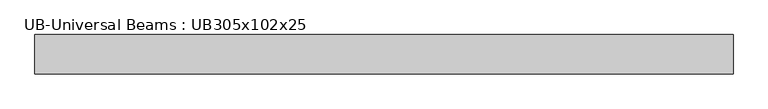
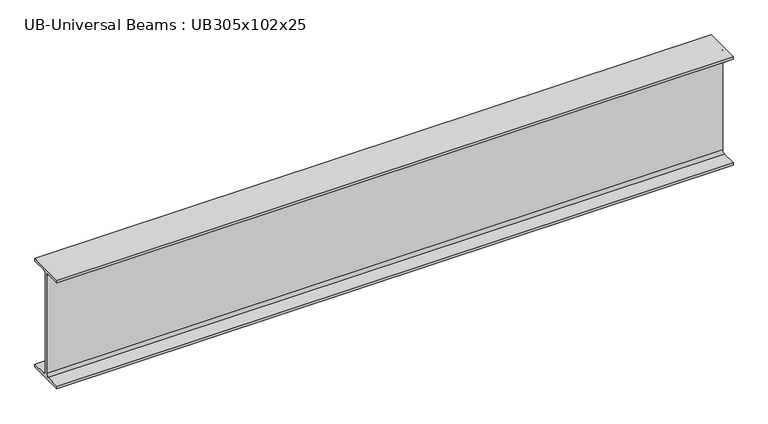
"""IFC4 building model written with IfcOpenShell, lengths in millimetres: beam geometry, UB-Universal Beams : UB305x102x25."""

from ifc_helpers import new_model, si_unit, point, frame, frame_2d, origin, place, context, project, spatial, polyline, circle_curve, trimmed, segment, composite_curve, outline, extrude, source, transform, mapped, element, save


def ub_universal_beams_ub305x102x25_e3bd1737(model_context):
    return source(origin(), model_context, "Body", "SweptSolid", [
        extrude(outline(composite_curve([segment(polyline([(50.8, -145.55), (50.8, -152.55), (-50.8, -152.55), (-50.8, -145.55), (-10.5, -145.55)]), True, "CONTINUOUS"), segment(trimmed(circle_curve(frame_2d((-10.5, -137.95)), 7.6), [point((-10.5, -145.55))], [point((-2.9, -137.95))], True, "CARTESIAN"), True, "CONTINUOUS"), segment(polyline([(-2.9, -137.95), (-2.9, 137.95)]), True, "CONTINUOUS"), segment(trimmed(circle_curve(frame_2d((-10.5, 137.95)), 7.6), [point((-2.9, 137.95))], [point((-10.5, 145.55))], True, "CARTESIAN"), True, "CONTINUOUS"), segment(polyline([(-10.5, 145.55), (-50.8, 145.55), (-50.8, 152.55), (50.8, 152.55), (50.8, 145.55), (10.5, 145.55)]), True, "CONTINUOUS"), segment(trimmed(circle_curve(frame_2d((10.5, 137.95)), 7.6), [point((10.5, 145.55))], [point((2.9, 137.95))], True, "CARTESIAN"), True, "CONTINUOUS"), segment(polyline([(2.9, 137.95), (2.9, -137.95)]), True, "CONTINUOUS"), segment(trimmed(circle_curve(frame_2d((10.5, -137.95)), 7.6), [point((2.9, -137.95))], [point((10.5, -145.55))], True, "CARTESIAN"), True, "CONTINUOUS"), segment(polyline([(10.5, -145.55), (50.8, -145.55)]), True, "CONTINUOUS")], self_intersect=False)), frame((-900.0, 0.0, 0.0), z_axis=(1.0, 0.0, 0.0), x_axis=(0.0, 1.0, 0.0)), (0.0, 0.0, 1.0), 1800.0),
    ])


if __name__ == "__main__":
    model = new_model("IFC4")
    model_context = context("Model", 3, world=origin())
    ifc_project = project(units=[si_unit("LENGTHUNIT", "METRE", prefix="MILLI")], contexts=[model_context])
    site = spatial("IfcSite", under=ifc_project)
    building = spatial("IfcBuilding", under=site)
    placement = place(None, origin())
    ub_universal_beams_ub305x102x25_shape = ub_universal_beams_ub305x102x25_e3bd1737(model_context)
    element("IfcBeam", 1, ObjectType="UB-Universal Beams : UB305x102x25", at=placement, inside=building, context=model_context, shape_type="MappedRepresentation", body=[
        mapped(ub_universal_beams_ub305x102x25_shape, transform((0.0, 0.0, 0.0), x_axis=(1.0, 0.0, 0.0), y_axis=(0.0, 1.0, 0.0), z_axis=(0.0, 0.0, 1.0))),
    ])
    save(model, "model.ifc")

# Revit data of these elements
# Type "UB-Universal Beams : UB305x102x25"
#   Section Name Key = "UB305X102X25"
#   Width = 10.16 cm
#   Web Thickness = 0.58 cm
#   Web Fillet = 0.76 cm
#   Warping Constant = 27300.0 cm⁶
#   Torsional Moment of Inertia = 4.77 cm⁴
#   Section Area = 31.6 cm²
#   Plastic Modulus weak axis = 39.0 cm³
#   Plastic Modulus strong axis = 342.0 cm³
#   Nominal Weight = 24.7999 kgf/m
#   Moment of Inertia weak axis = 123.00 cm⁴
#   Moment of Inertia strong axis = 4455.00 cm⁴
#   Height = 30.51 cm
#   Flange Thickness = 0.7 cm
#   Elastic Modulus weak axis = 24.2 cm³
#   Elastic Modulus strong axis = 292.0 cm³
#   Centroid Vertical = 15.255 cm
#   Centroid Horizontal = 5.08 cm
#   Bolt Spacing = 5.4 cm
#   Length [instance default] = 1.5 m
#   Structural Material [instance default] = Metal - Steel 43-275
#   Type Comments = ""
#   Assembly Code = ""
# Element 1 (IfcBeam, "UB-Universal Beams : UB305x102x25")
#   Materials on its faces: "Metal - Steel 43-275"
# Materials
#   "Metal - Steel 43-275": class "Metal", colour RGB 247 247 247, transparency 0, Cost = 0
